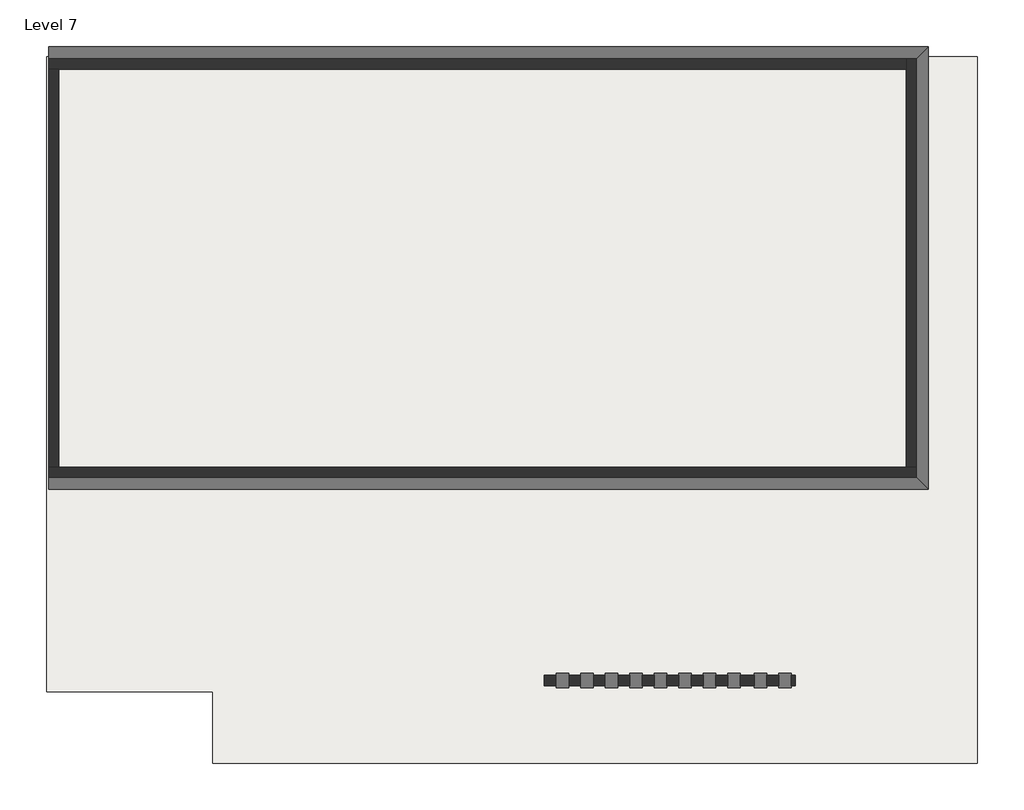
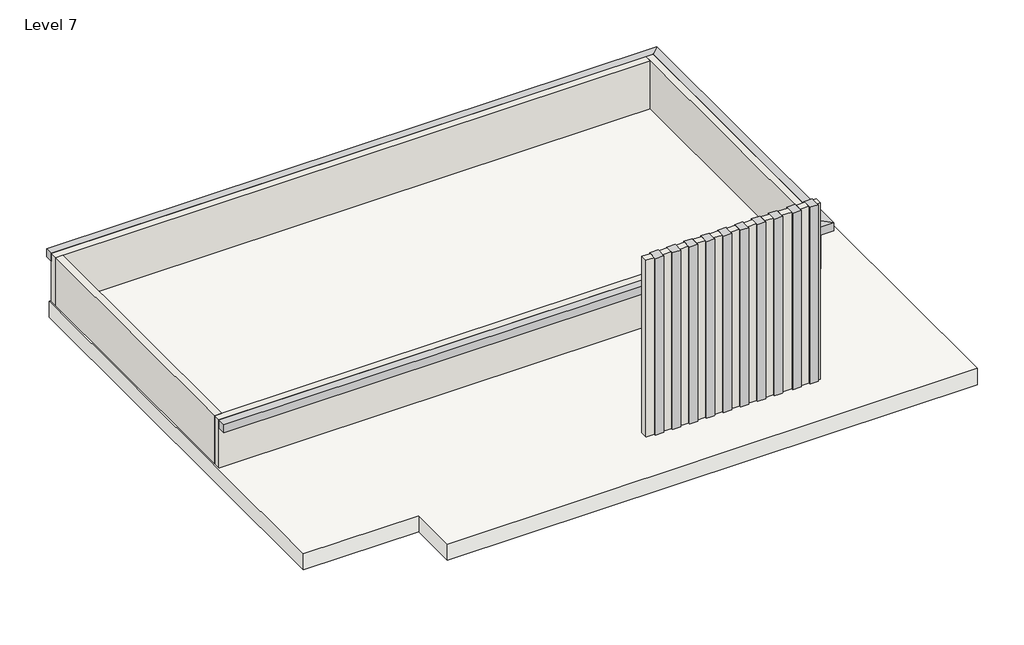
# One storey: 13 proxies, 5 walls, 1 roof.
"""IFC4 building model written with IfcOpenShell, lengths in millimetres."""

from ifc_helpers import new_model, si_unit, frame, origin, place, context, project, spatial, polyline, outline, extrude, faceted_brep, element, save

model = new_model("IFC4")

# Units and contexts
model_context = context("Model", 3, world=origin())
ifc_project = project(units=[si_unit("LENGTHUNIT", "METRE", prefix="MILLI")], contexts=[model_context])

# Site, building, storey
site = spatial("IfcSite", under=ifc_project)
building = spatial("IfcBuilding", under=site)
storey = spatial("IfcBuildingStorey", under=building, Name="Level 7", Elevation=21945.6)

# Proxies
placement = place(None, origin())
element("IfcBuildingElementProxy", 1, Name="Cornice", ObjectType="Cornice", at=placement, inside=storey, context=model_context, shape_type="SweptSolid", body=[
    extrude(outline(polyline([(-14184.3864811, 5574.2732783), (-14184.3864811, 5726.6732783), (-3389.3864811, 5726.6732783), (-3236.9864811, 5574.2732783), (-14184.3864811, 5574.2732783)])), frame((0.0, 0.0, 23012.4), z_axis=(0.0, 0.0, 1.0), x_axis=(1.0, 0.0, 0.0)), (0.0, 0.0, 1.0), 152.4),
])
element("IfcBuildingElementProxy", 2, Name="Cornice", ObjectType="Cornice", at=placement, inside=storey, context=model_context, shape_type="SweptSolid", body=[
    extrude(outline(polyline([(-3236.9864811, 5574.2732783), (-3389.3864811, 5726.6732783), (-3389.3864811, 10932.8297737), (-3236.9864811, 11085.2297737), (-3236.9864811, 5574.2732783)])), frame((0.0, 0.0, 23012.4), z_axis=(0.0, 0.0, 1.0), x_axis=(1.0, 0.0, 0.0)), (0.0, 0.0, 1.0), 152.4),
])
element("IfcBuildingElementProxy", 3, Name="Cornice", ObjectType="Cornice", at=placement, inside=storey, context=model_context, shape_type="SweptSolid", body=[
    extrude(outline(polyline([(-3236.9864811, 11085.2297737), (-3389.3864811, 10932.8297737), (-14184.3864811, 10932.8297737), (-14184.3864811, 11085.2297737), (-3236.9864811, 11085.2297737)])), frame((0.0, 0.0, 23012.4), z_axis=(0.0, 0.0, 1.0), x_axis=(1.0, 0.0, 0.0)), (0.0, 0.0, 1.0), 152.4),
])
element("IfcBuildingElementProxy", 4, Name="Reveal", ObjectType="Reveal", at=placement, inside=storey, context=model_context, shape_type="SweptSolid", body=[
    extrude(outline(polyline([(-7865.7304753, 3104.5497737), (-7865.7304753, 3287.4297737), (-7713.3304753, 3287.4297737), (-7713.3304753, 3104.5497737), (-7865.7304753, 3104.5497737)])), frame((0.0, 0.0, 22250.4), z_axis=(0.0, 0.0, 1.0), x_axis=(1.0, 0.0, 0.0)), (0.0, 0.0, 1.0), 3352.8),
])
element("IfcBuildingElementProxy", 5, Name="Reveal", ObjectType="Reveal", at=placement, inside=storey, context=model_context, shape_type="SweptSolid", body=[
    extrude(outline(polyline([(-7560.9304753, 3104.5497737), (-7560.9304753, 3287.4297737), (-7408.5304753, 3287.4297737), (-7408.5304753, 3104.5497737), (-7560.9304753, 3104.5497737)])), frame((0.0, 0.0, 22250.4), z_axis=(0.0, 0.0, 1.0), x_axis=(1.0, 0.0, 0.0)), (0.0, 0.0, 1.0), 3352.8),
])
element("IfcBuildingElementProxy", 6, Name="Reveal", ObjectType="Reveal", at=placement, inside=storey, context=model_context, shape_type="SweptSolid", body=[
    extrude(outline(polyline([(-7256.1304753, 3104.5497737), (-7256.1304753, 3287.4297737), (-7103.7304753, 3287.4297737), (-7103.7304753, 3104.5497737), (-7256.1304753, 3104.5497737)])), frame((0.0, 0.0, 22250.4), z_axis=(0.0, 0.0, 1.0), x_axis=(1.0, 0.0, 0.0)), (0.0, 0.0, 1.0), 3352.8),
])
element("IfcBuildingElementProxy", 7, Name="Reveal", ObjectType="Reveal", at=placement, inside=storey, context=model_context, shape_type="SweptSolid", body=[
    extrude(outline(polyline([(-6951.3304753, 3104.5497737), (-6951.3304753, 3287.4297737), (-6798.9304753, 3287.4297737), (-6798.9304753, 3104.5497737), (-6951.3304753, 3104.5497737)])), frame((0.0, 0.0, 22250.4), z_axis=(0.0, 0.0, 1.0), x_axis=(1.0, 0.0, 0.0)), (0.0, 0.0, 1.0), 3352.8),
])
element("IfcBuildingElementProxy", 8, Name="Reveal", ObjectType="Reveal", at=placement, inside=storey, context=model_context, shape_type="SweptSolid", body=[
    extrude(outline(polyline([(-6646.5304753, 3104.5497737), (-6646.5304753, 3287.4297737), (-6494.1304753, 3287.4297737), (-6494.1304753, 3104.5497737), (-6646.5304753, 3104.5497737)])), frame((0.0, 0.0, 22250.4), z_axis=(0.0, 0.0, 1.0), x_axis=(1.0, 0.0, 0.0)), (0.0, 0.0, 1.0), 3352.8),
])
element("IfcBuildingElementProxy", 9, Name="Reveal", ObjectType="Reveal", at=placement, inside=storey, context=model_context, shape_type="SweptSolid", body=[
    extrude(outline(polyline([(-6341.7304753, 3104.5497737), (-6341.7304753, 3287.4297737), (-6189.3304753, 3287.4297737), (-6189.3304753, 3104.5497737), (-6341.7304753, 3104.5497737)])), frame((0.0, 0.0, 22250.4), z_axis=(0.0, 0.0, 1.0), x_axis=(1.0, 0.0, 0.0)), (0.0, 0.0, 1.0), 3352.8),
])
element("IfcBuildingElementProxy", 10, Name="Reveal", ObjectType="Reveal", at=placement, inside=storey, context=model_context, shape_type="SweptSolid", body=[
    extrude(outline(polyline([(-6036.9304753, 3104.5497737), (-6036.9304753, 3287.4297737), (-5884.5304753, 3287.4297737), (-5884.5304753, 3104.5497737), (-6036.9304753, 3104.5497737)])), frame((0.0, 0.0, 22250.4), z_axis=(0.0, 0.0, 1.0), x_axis=(1.0, 0.0, 0.0)), (0.0, 0.0, 1.0), 3352.8),
])
element("IfcBuildingElementProxy", 11, Name="Reveal", ObjectType="Reveal", at=placement, inside=storey, context=model_context, shape_type="SweptSolid", body=[
    extrude(outline(polyline([(-5732.1304753, 3104.5497737), (-5732.1304753, 3287.4297737), (-5579.7304753, 3287.4297737), (-5579.7304753, 3104.5497737), (-5732.1304753, 3104.5497737)])), frame((0.0, 0.0, 22250.4), z_axis=(0.0, 0.0, 1.0), x_axis=(1.0, 0.0, 0.0)), (0.0, 0.0, 1.0), 3352.8),
])
element("IfcBuildingElementProxy", 12, Name="Reveal", ObjectType="Reveal", at=placement, inside=storey, context=model_context, shape_type="SweptSolid", body=[
    extrude(outline(polyline([(-5401.9304753, 3104.5497737), (-5401.9304753, 3287.4297737), (-5249.5304753, 3287.4297737), (-5249.5304753, 3104.5497737), (-5401.9304753, 3104.5497737)])), frame((0.0, 0.0, 22250.4), z_axis=(0.0, 0.0, 1.0), x_axis=(1.0, 0.0, 0.0)), (0.0, 0.0, 1.0), 3352.8),
])
element("IfcBuildingElementProxy", 13, Name="Reveal", ObjectType="Reveal", at=placement, inside=storey, context=model_context, shape_type="SweptSolid", body=[
    extrude(outline(polyline([(-5097.1304753, 3104.5497737), (-5097.1304753, 3287.4297737), (-4944.7304753, 3287.4297737), (-4944.7304753, 3104.5497737), (-5097.1304753, 3104.5497737)])), frame((0.0, 0.0, 22250.4), z_axis=(0.0, 0.0, 1.0), x_axis=(1.0, 0.0, 0.0)), (0.0, 0.0, 1.0), 3352.8),
])

# Roof
element("IfcRoof", 14, ObjectType="Generic - 12\"", at=placement, inside=storey, context=model_context, shape_type="SweptSolid", body=[
    extrude(outline(polyline([(-14209.7864811, 10958.2297737), (-2627.3864811, 10958.2297737), (-2627.3864811, 2169.8297737), (-12139.2804753, 2169.8297737), (-12139.2804753, 3058.8297737), (-14209.7864811, 3058.8297737), (-14209.7864811, 10958.2297737)])), frame((0.0, 0.0, 21945.6), z_axis=(0.0, 0.0, 1.0), x_axis=(1.0, 0.0, 0.0)), (0.0, 0.0, 1.0), 304.8),
])

# Walls
element("IfcWall", 15, ObjectType="Generic - 5\"", at=placement, inside=storey, context=model_context, shape_type="SweptSolid", body=[
    extrude(outline(polyline([(-8018.1304753, 3135.0297737), (-8018.1304753, 3262.0297737), (-7865.7304753, 3262.0297737), (-7865.7304753, 3135.0297737), (-8018.1304753, 3135.0297737)])), frame((0.0, 0.0, 22250.4), z_axis=(0.0, 0.0, 1.0), x_axis=(1.0, 0.0, 0.0)), (0.0, 0.0, 1.0), 3352.8),
    extrude(outline(polyline([(-4893.9304753, 3262.0297737), (-4893.9304753, 3135.0297737), (-4944.7304753, 3135.0297737), (-4944.7304753, 3262.0297737), (-4893.9304753, 3262.0297737)])), frame((0.0, 0.0, 22250.4), z_axis=(0.0, 0.0, 1.0), x_axis=(1.0, 0.0, 0.0)), (0.0, 0.0, 1.0), 3352.8),
    extrude(outline(polyline([(-7713.3304753, 3135.0297737), (-7713.3304753, 3262.0297737), (-7560.9304753, 3262.0297737), (-7560.9304753, 3135.0297737), (-7713.3304753, 3135.0297737)])), frame((0.0, 0.0, 22250.4), z_axis=(0.0, 0.0, 1.0), x_axis=(1.0, 0.0, 0.0)), (0.0, 0.0, 1.0), 3352.8),
    extrude(outline(polyline([(-7408.5304753, 3135.0297737), (-7408.5304753, 3262.0297737), (-7256.1304753, 3262.0297737), (-7256.1304753, 3135.0297737), (-7408.5304753, 3135.0297737)])), frame((0.0, 0.0, 22250.4), z_axis=(0.0, 0.0, 1.0), x_axis=(1.0, 0.0, 0.0)), (0.0, 0.0, 1.0), 3352.8),
    extrude(outline(polyline([(-7103.7304753, 3135.0297737), (-7103.7304753, 3262.0297737), (-6951.3304753, 3262.0297737), (-6951.3304753, 3135.0297737), (-7103.7304753, 3135.0297737)])), frame((0.0, 0.0, 22250.4), z_axis=(0.0, 0.0, 1.0), x_axis=(1.0, 0.0, 0.0)), (0.0, 0.0, 1.0), 3352.8),
    extrude(outline(polyline([(-6798.9304753, 3135.0297737), (-6798.9304753, 3262.0297737), (-6646.5304753, 3262.0297737), (-6646.5304753, 3135.0297737), (-6798.9304753, 3135.0297737)])), frame((0.0, 0.0, 22250.4), z_axis=(0.0, 0.0, 1.0), x_axis=(1.0, 0.0, 0.0)), (0.0, 0.0, 1.0), 3352.8),
    extrude(outline(polyline([(-6494.1304753, 3135.0297737), (-6494.1304753, 3262.0297737), (-6341.7304753, 3262.0297737), (-6341.7304753, 3135.0297737), (-6494.1304753, 3135.0297737)])), frame((0.0, 0.0, 22250.4), z_axis=(0.0, 0.0, 1.0), x_axis=(1.0, 0.0, 0.0)), (0.0, 0.0, 1.0), 3352.8),
    extrude(outline(polyline([(-6189.3304753, 3135.0297737), (-6189.3304753, 3262.0297737), (-6036.9304753, 3262.0297737), (-6036.9304753, 3135.0297737), (-6189.3304753, 3135.0297737)])), frame((0.0, 0.0, 22250.4), z_axis=(0.0, 0.0, 1.0), x_axis=(1.0, 0.0, 0.0)), (0.0, 0.0, 1.0), 3352.8),
    extrude(outline(polyline([(-5884.5304753, 3135.0297737), (-5884.5304753, 3262.0297737), (-5732.1304753, 3262.0297737), (-5732.1304753, 3135.0297737), (-5884.5304753, 3135.0297737)])), frame((0.0, 0.0, 22250.4), z_axis=(0.0, 0.0, 1.0), x_axis=(1.0, 0.0, 0.0)), (0.0, 0.0, 1.0), 3352.8),
    extrude(outline(polyline([(-5579.7304753, 3135.0297737), (-5579.7304753, 3262.0297737), (-5401.9304753, 3262.0297737), (-5401.9304753, 3135.0297737), (-5579.7304753, 3135.0297737)])), frame((0.0, 0.0, 22250.4), z_axis=(0.0, 0.0, 1.0), x_axis=(1.0, 0.0, 0.0)), (0.0, 0.0, 1.0), 3352.8),
    extrude(outline(polyline([(-5249.5304753, 3135.0297737), (-5249.5304753, 3262.0297737), (-5097.1304753, 3262.0297737), (-5097.1304753, 3135.0297737), (-5249.5304753, 3135.0297737)])), frame((0.0, 0.0, 22250.4), z_axis=(0.0, 0.0, 1.0), x_axis=(1.0, 0.0, 0.0)), (0.0, 0.0, 1.0), 3352.8),
])
element("IfcWall", 16, ObjectType="Generic - 5\"", at=placement, inside=storey, context=model_context, shape_type="Brep", body=[
    faceted_brep([(-14184.3864811, 5726.6732783, 21945.6), (-3389.3864811, 5726.6732783, 21945.6), (-3389.3864811, 5726.6732783, 23164.8), (-14184.3864811, 5726.6732783, 23164.8), (-14184.3864811, 5853.6732783, 21945.6), (-14184.3864811, 5853.6732783, 23164.8), (-14057.3864811, 5853.6732783, 23164.8), (-3516.3864811, 5853.6732783, 23164.8), (-3389.3864811, 5853.6732783, 23164.8), (-3389.3864811, 5853.6732783, 21945.6), (-3516.3864811, 5853.6732783, 21945.6), (-14057.3864811, 5853.6732783, 21945.6)], [[[0, 1, 2, 3]], [[4, 5, 6, 7, 8, 9, 10, 11]], [[1, 0, 4, 11, 10, 9]], [[3, 2, 8, 7, 6, 5]], [[2, 1, 9, 8]], [[0, 3, 5, 4]]]),
])
element("IfcWall", 17, ObjectType="Generic - 5\"", at=placement, inside=storey, context=model_context, shape_type="Brep", body=[
    faceted_brep([(-3389.3864811, 5853.6732783, 21945.6), (-3389.3864811, 10932.8297737, 21945.6), (-3389.3864811, 10932.8297737, 23012.4), (-3389.3864811, 10932.8297737, 23164.8), (-3389.3864811, 5853.6732783, 23164.8), (-3389.3864811, 5853.6732783, 23012.4), (-3516.3864811, 10932.8297737, 21945.6), (-3516.3864811, 10805.8297737, 21945.6), (-3516.3864811, 5853.6732783, 21945.6), (-3516.3864811, 5853.6732783, 23164.8), (-3516.3864811, 10805.8297737, 23164.8), (-3516.3864811, 10932.8297737, 23164.8), (-3516.3864811, 10932.8297737, 23012.4)], [[[0, 1, 2, 3, 4, 5]], [[6, 7, 8, 9, 10, 11, 12]], [[1, 0, 8, 7, 6]], [[4, 3, 11, 10, 9]], [[4, 9, 8, 0, 5]], [[1, 6, 12, 11, 3, 2]]]),
])
element("IfcWall", 18, ObjectType="Generic - 5\"", at=placement, inside=storey, context=model_context, shape_type="Brep", body=[
    faceted_brep([(-3516.3864811, 10932.8297737, 21945.6), (-14184.3864811, 10932.8297737, 21945.6), (-14184.3864811, 10932.8297737, 23012.4), (-14184.3864811, 10932.8297737, 23164.8), (-3516.3864811, 10932.8297737, 23164.8), (-3516.3864811, 10932.8297737, 23012.4), (-14184.3864811, 10805.8297737, 21945.6), (-14057.3864811, 10805.8297737, 21945.6), (-3516.3864811, 10805.8297737, 21945.6), (-3516.3864811, 10805.8297737, 23164.8), (-14057.3864811, 10805.8297737, 23164.8), (-14184.3864811, 10805.8297737, 23164.8)], [[[0, 1, 2, 3, 4, 5]], [[6, 7, 8, 9, 10, 11]], [[1, 0, 8, 7, 6]], [[4, 3, 11, 10, 9]], [[4, 9, 8, 0, 5]], [[1, 6, 11, 3, 2]]]),
])
element("IfcWall", 19, ObjectType="Generic - 5\"", at=placement, inside=storey, context=model_context, shape_type="SweptSolid", body=[
    extrude(outline(polyline([(-14184.3864811, 5853.6732783), (-14184.3864811, 10805.8297737), (-14057.3864811, 10805.8297737), (-14057.3864811, 5853.6732783), (-14184.3864811, 5853.6732783)])), frame((0.0, 0.0, 21945.6), z_axis=(0.0, 0.0, 1.0), x_axis=(1.0, 0.0, 0.0)), (0.0, 0.0, 1.0), 1219.2),
])

save(model, "model.ifc")

# Revit data of these elements
# Type "Generic - 12\""
#   Assembly Code = "B1020"
#   Layers, outside or top first: 1' - 0" no material (function 1)
# Type "Generic - 5\""
#   Assembly Code = "B2010"
#   Layers, outside or top first: 0' - 5" no material (function 1)
# Elements 1, 2, 3 (IfcBuildingElementProxy, "Cornice")
#   Phase Created = New Construction
#   Materials on its faces: "Default Wall"
# Element 14 (IfcRoof, "Generic - 12\"")
#   built-in parameter 1001705 = 73 (stored number, unit not read)
#   built-in parameter 1001710 = 33615
#   Phase Created = New Construction
#   Materials on its faces: "Default Roof"
# Element 15 (IfcWall, "Generic - 5\"")
#   built-in parameter 1001111 = 1' - 0"
#   Top Offset = 0' - 0"
#   Base Offset = 1' - 0"
#   wall height = 11' - 0"
#   Phase Created = New Construction
#   Base Constraint = Level 7
#   Top Constraint = Level 8
#   Materials on its faces: "Default Wall"
# Elements 16, 17, 18, 19 (IfcWall, "Generic - 5\"")
#   Top Offset = -8' - 0"
#   Base Offset = 0' - 0"
#   wall height = 4' - 0"
#   Phase Created = New Construction
#   Base Constraint = Level 7
#   Top Constraint = Level 8
#   Materials on its faces: "Default Wall"
# Materials
#   "Default Wall": colour RGB 128 128 128, transparency 0
#   "Default Roof": colour RGB 88 101 114, transparency 0
